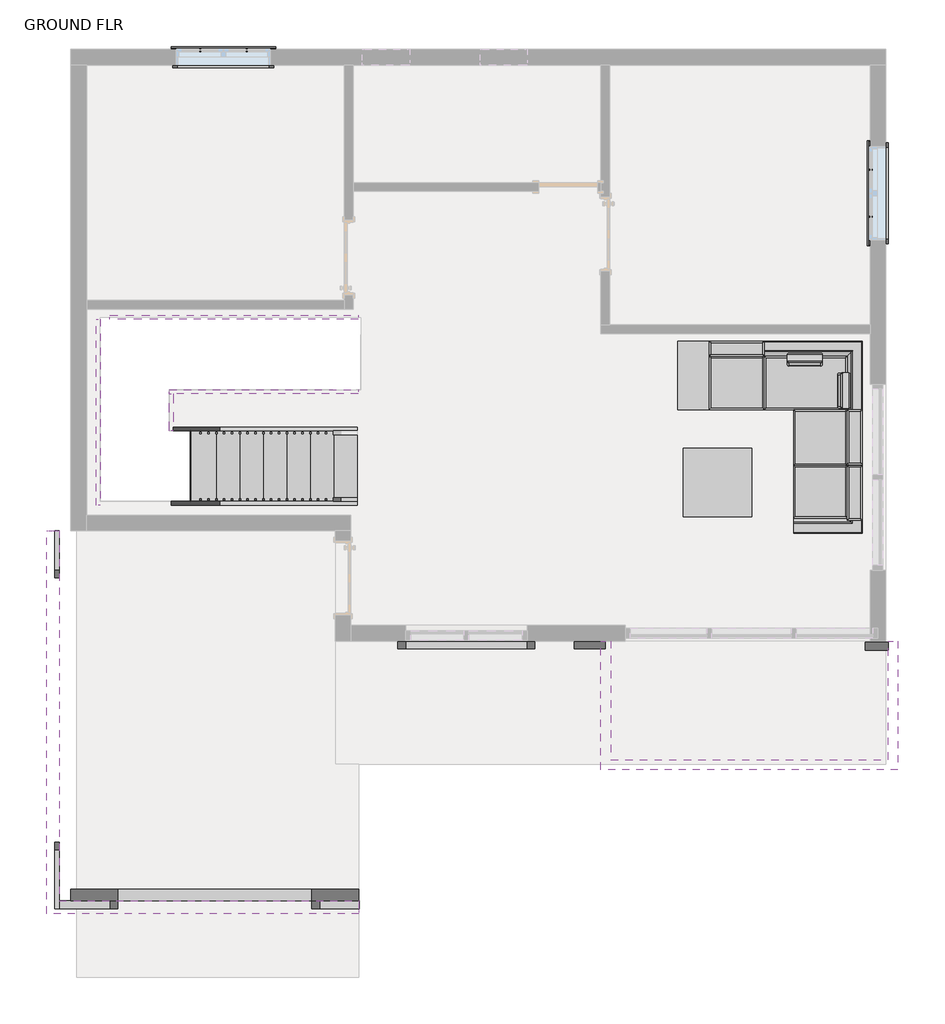
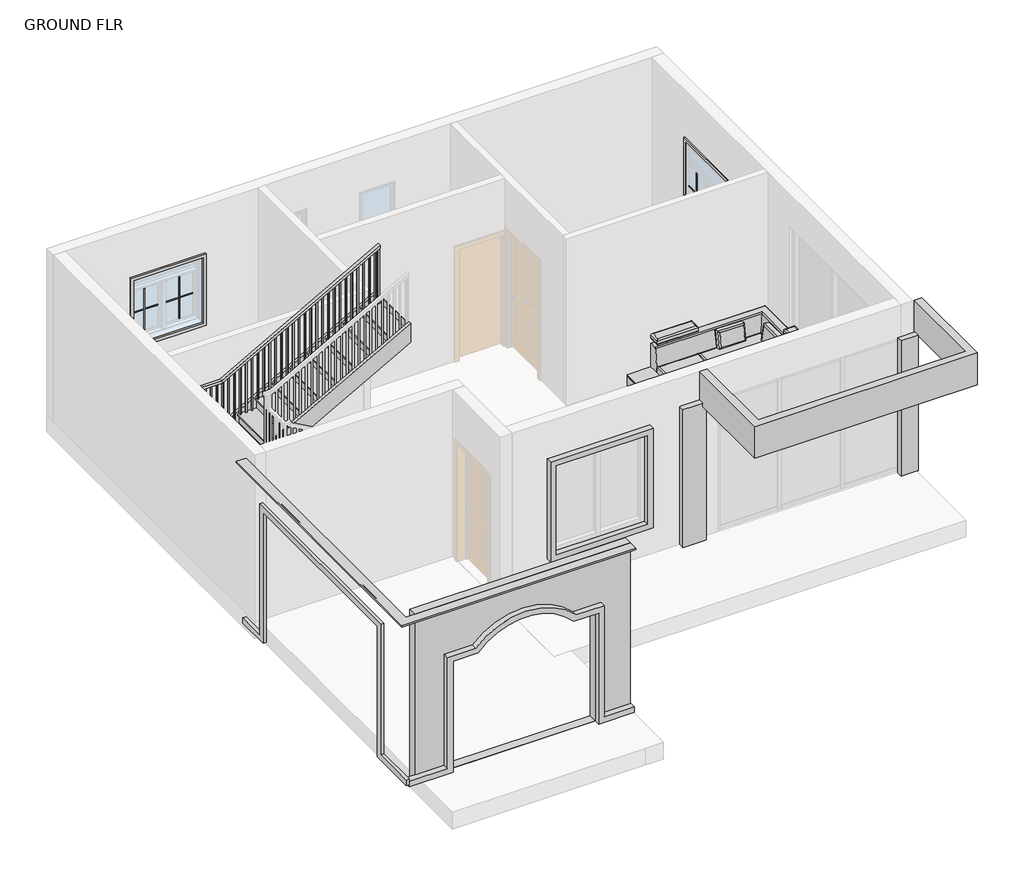
# One storey, part 3 of 3: 17 proxies, 6 members, 1 railing, 1 stair flight.
"""IFC4 building model written with IfcOpenShell, lengths in millimetres."""

from ifc_helpers import new_model, si_unit, frame, origin, place, context, project, spatial, polyline, outline, extrude, faceted_brep, transform, mapped, element, save
from components import generic_models_1_generic_models_1_99b3fc70, generic_models_10_generic_models_10_d7661e71, generic_models_11_generic_models_11_c52e9c8d, generic_models_2_generic_models_2_85994228, generic_models_3_generic_models_3_794cf474, generic_models_4_generic_models_4_3df0761b, generic_models_7_generic_models_7_ebfadceb, generic_models_9_generic_models_9_ba76ca7f, muntin_pattern_2x2_muntin_pattern_2x2_2357e71d, muntin_pattern_2x2_muntin_pattern_2x2_302d8f29, trim_window_exterior_flat_with_sill_7cfdd449, trim_window_exterior_flat_with_sill_ac84ebb5, trim_window_interior_flat_picture_frame_f1e0b15b, trim_window_interior_flat_picture_frame_caf2db4f, sectional_sofa_6482_sectional_sofa_6482_559db2f0, sectional_sofa_6482_sectional_sofa_6482_9496661e, stair_flight_1ef6648f

model = new_model("IFC4")

# Units and contexts
model_context = context("Model", 3, world=origin())
ifc_project = project(units=[si_unit("LENGTHUNIT", "METRE", prefix="MILLI")], contexts=[model_context])

# Site, building, storey
site = spatial("IfcSite", under=ifc_project)
building = spatial("IfcBuilding", under=site)
storey = spatial("IfcBuildingStorey", under=building, Name="GROUND FLR", Elevation=304.8)

# Proxies
placement = place(None, origin())
generic_models_1_generic_models_1_shape = generic_models_1_generic_models_1_99b3fc70(model_context)
element("IfcBuildingElementProxy", 1, Name="Generic Models 1 : Generic Models 1", ObjectType="Generic Models 1 : Generic Models 1", at=placement, inside=storey, context=model_context, shape_type="MappedRepresentation", body=[
    mapped(generic_models_1_generic_models_1_shape, transform((0.0, 0.0, 0.0), x_axis=(1.0, 0.0, 0.0), y_axis=(0.0, 1.0, 0.0), z_axis=(0.0, 0.0, 1.0))),
])
generic_models_10_generic_models_10_shape = generic_models_10_generic_models_10_d7661e71(model_context)
element("IfcBuildingElementProxy", 2, Name="Generic Models 10 : Generic Models 10", ObjectType="Generic Models 10 : Generic Models 10", at=placement, inside=storey, context=model_context, shape_type="MappedRepresentation", body=[
    mapped(generic_models_10_generic_models_10_shape, transform((0.0, 0.0, 0.0), x_axis=(1.0, 0.0, 0.0), y_axis=(0.0, 1.0, 0.0), z_axis=(0.0, 0.0, 1.0))),
])
generic_models_11_generic_models_11_shape = generic_models_11_generic_models_11_c52e9c8d(model_context)
element("IfcBuildingElementProxy", 3, Name="Generic Models 11 : Generic Models 11", ObjectType="Generic Models 11 : Generic Models 11", at=placement, inside=storey, context=model_context, shape_type="MappedRepresentation", body=[
    mapped(generic_models_11_generic_models_11_shape, transform((0.0, 0.0, 0.0), x_axis=(1.0, 0.0, 0.0), y_axis=(0.0, 1.0, 0.0), z_axis=(0.0, 0.0, 1.0))),
])
generic_models_2_generic_models_2_shape = generic_models_2_generic_models_2_85994228(model_context)
element("IfcBuildingElementProxy", 4, Name="Generic Models 2 : Generic Models 2", ObjectType="Generic Models 2 : Generic Models 2", at=placement, inside=storey, context=model_context, shape_type="MappedRepresentation", body=[
    mapped(generic_models_2_generic_models_2_shape, transform((0.0, 0.0, 0.0), x_axis=(1.0, 0.0, 0.0), y_axis=(0.0, 1.0, 0.0), z_axis=(0.0, 0.0, 1.0))),
])
generic_models_3_generic_models_3_shape = generic_models_3_generic_models_3_794cf474(model_context)
element("IfcBuildingElementProxy", 5, Name="Generic Models 3 : Generic Models 3", ObjectType="Generic Models 3 : Generic Models 3", at=placement, inside=storey, context=model_context, shape_type="MappedRepresentation", body=[
    mapped(generic_models_3_generic_models_3_shape, transform((0.0, 0.0, 0.0), x_axis=(1.0, 0.0, 0.0), y_axis=(0.0, 1.0, 0.0), z_axis=(0.0, 0.0, 1.0))),
])
generic_models_4_generic_models_4_shape = generic_models_4_generic_models_4_3df0761b(model_context)
element("IfcBuildingElementProxy", 6, Name="Generic Models 4 : Generic Models 4", ObjectType="Generic Models 4 : Generic Models 4", at=placement, inside=storey, context=model_context, shape_type="MappedRepresentation", body=[
    mapped(generic_models_4_generic_models_4_shape, transform((0.0, 0.0, 0.0), x_axis=(1.0, 0.0, 0.0), y_axis=(0.0, 1.0, 0.0), z_axis=(0.0, 0.0, 1.0))),
])
generic_models_7_generic_models_7_shape = generic_models_7_generic_models_7_ebfadceb(model_context)
element("IfcBuildingElementProxy", 7, Name="Generic Models 7 : Generic Models 7", ObjectType="Generic Models 7 : Generic Models 7", at=placement, inside=storey, context=model_context, shape_type="MappedRepresentation", body=[
    mapped(generic_models_7_generic_models_7_shape, transform((0.0, 0.0, 0.0), x_axis=(1.0, 0.0, 0.0), y_axis=(0.0, 1.0, 0.0), z_axis=(0.0, 0.0, 1.0))),
])
generic_models_9_generic_models_9_shape = generic_models_9_generic_models_9_ba76ca7f(model_context)
element("IfcBuildingElementProxy", 8, Name="Generic Models 9 : Generic Models 9", ObjectType="Generic Models 9 : Generic Models 9", at=placement, inside=storey, context=model_context, shape_type="MappedRepresentation", body=[
    mapped(generic_models_9_generic_models_9_shape, transform((0.0, 0.0, 0.0), x_axis=(1.0, 0.0, 0.0), y_axis=(0.0, 1.0, 0.0), z_axis=(0.0, 0.0, 1.0))),
])
muntin_pattern_2x2_muntin_pattern_2x2_shape = muntin_pattern_2x2_muntin_pattern_2x2_2357e71d(model_context)
element("IfcBuildingElementProxy", 9, Name="Muntin Pattern_2x2 : Muntin Pattern_2x2", ObjectType="Muntin Pattern_2x2 : Muntin Pattern_2x2", at=placement, inside=storey, context=model_context, shape_type="MappedRepresentation", body=[
    mapped(muntin_pattern_2x2_muntin_pattern_2x2_shape, transform((-9970.7895642, -2610.1146616, 1289.05), x_axis=(1.0, 0.0, 0.0), y_axis=(0.0, 1.0, 0.0), z_axis=(0.0, 0.0, 1.0))),
])
element("IfcBuildingElementProxy", 10, Name="Muntin Pattern_2x2 : Muntin Pattern_2x2", ObjectType="Muntin Pattern_2x2 : Muntin Pattern_2x2", at=placement, inside=storey, context=model_context, shape_type="MappedRepresentation", body=[
    mapped(muntin_pattern_2x2_muntin_pattern_2x2_shape, transform((-1272.9986584, -4768.3196866, 1289.05), x_axis=(0.0, 1.0, 0.0), y_axis=(-1.0, 0.0, 0.0), z_axis=(0.0, 0.0, 1.0))),
])
muntin_pattern_2x2_muntin_pattern_2x2_2_shape = muntin_pattern_2x2_muntin_pattern_2x2_302d8f29(model_context)
element("IfcBuildingElementProxy", 11, Name="Muntin Pattern_2x2 : Muntin Pattern_2x2", ObjectType="Muntin Pattern_2x2 : Muntin Pattern_2x2", at=placement, inside=storey, context=model_context, shape_type="MappedRepresentation", body=[
    mapped(muntin_pattern_2x2_muntin_pattern_2x2_2_shape, transform((-9364.3645642, -2610.1146616, 1289.05), x_axis=(-1.0, 0.0, 0.0), y_axis=(0.0, -1.0, 0.0), z_axis=(0.0, 0.0, 1.0))),
])
element("IfcBuildingElementProxy", 12, Name="Muntin Pattern_2x2 : Muntin Pattern_2x2", ObjectType="Muntin Pattern_2x2 : Muntin Pattern_2x2", at=placement, inside=storey, context=model_context, shape_type="MappedRepresentation", body=[
    mapped(muntin_pattern_2x2_muntin_pattern_2x2_2_shape, transform((-1272.9986584, -4161.8946866, 1289.05), x_axis=(0.0, -1.0, 0.0), y_axis=(1.0, 0.0, 0.0), z_axis=(0.0, 0.0, 1.0))),
])
trim_window_exterior_flat_with_sill_shape = trim_window_exterior_flat_with_sill_7cfdd449(model_context)
element("IfcBuildingElementProxy", 13, Name="Trim-Window-Exterior-Flat : with Sill", ObjectType="Trim-Window-Exterior-Flat : with Sill", at=placement, inside=storey, context=model_context, shape_type="MappedRepresentation", body=[
    mapped(trim_window_exterior_flat_with_sill_shape, transform((-9667.5770642, -2600.5896616, 2438.4), x_axis=(-1.0, 0.0, 0.0), y_axis=(0.0, 0.0, 1.0), z_axis=(0.0, 1.0, 0.0))),
])
trim_window_exterior_flat_with_sill_2_shape = trim_window_exterior_flat_with_sill_ac84ebb5(model_context)
element("IfcBuildingElementProxy", 14, Name="Trim-Window-Exterior-Flat : with Sill", ObjectType="Trim-Window-Exterior-Flat : with Sill", at=placement, inside=storey, context=model_context, shape_type="MappedRepresentation", body=[
    mapped(trim_window_exterior_flat_with_sill_2_shape, transform((-1282.5236584, -4465.1071866, 2438.4), x_axis=(0.0, 1.0, 0.0), y_axis=(0.0, 0.0, -1.0), z_axis=(-1.0, 0.0, 0.0))),
])
trim_window_interior_flat_picture_frame_shape = trim_window_interior_flat_picture_frame_f1e0b15b(model_context)
element("IfcBuildingElementProxy", 15, Name="Trim-Window-Interior-Flat : Picture Frame", ObjectType="Trim-Window-Interior-Flat : Picture Frame", at=placement, inside=storey, context=model_context, shape_type="MappedRepresentation", body=[
    mapped(trim_window_interior_flat_picture_frame_shape, transform((-9667.5770642, -2803.7896616, 2438.4), x_axis=(1.0, 0.0, 0.0), y_axis=(0.0, 0.0, 1.0), z_axis=(0.0, -1.0, 0.0))),
])
trim_window_interior_flat_picture_frame_2_shape = trim_window_interior_flat_picture_frame_caf2db4f(model_context)
element("IfcBuildingElementProxy", 16, Name="Trim-Window-Interior-Flat : Picture Frame", ObjectType="Trim-Window-Interior-Flat : Picture Frame", at=placement, inside=storey, context=model_context, shape_type="MappedRepresentation", body=[
    mapped(trim_window_interior_flat_picture_frame_2_shape, transform((-1079.3236584, -4465.1071866, 2438.4), x_axis=(0.0, -1.0, 0.0), y_axis=(0.0, 0.0, -1.0), z_axis=(1.0, 0.0, 0.0))),
])
sectional_sofa_6482_sectional_sofa_6482_shape = sectional_sofa_6482_sectional_sofa_6482_559db2f0(model_context)
sectional_sofa_6482_sectional_sofa_6482_2_shape = sectional_sofa_6482_sectional_sofa_6482_9496661e(model_context)
element("IfcBuildingElementProxy", 17, Name="sectional_sofa_6482 : sectional_sofa_6482", ObjectType="sectional_sofa_6482 : sectional_sofa_6482", at=placement, inside=storey, context=model_context, shape_type="MappedRepresentation", body=[
    mapped(sectional_sofa_6482_sectional_sofa_6482_shape, transform((-2654.1236584, -7674.2396616, 304.8), x_axis=(1.0, 0.0, 0.0), y_axis=(0.0, 1.0, 0.0), z_axis=(0.0, 0.0, 1.0))),
    mapped(sectional_sofa_6482_sectional_sofa_6482_2_shape, transform((-2654.1236584, -7674.2396616, 304.8), x_axis=(1.0, 0.0, 0.0), y_axis=(0.0, 1.0, 0.0), z_axis=(0.0, 0.0, 1.0))),
])

# Members
element("IfcMember", 18, ObjectType="Stringer - 2\" Width", at=placement, inside=storey, context=model_context, shape_type="SweptSolid", body=[
    extrude(outline(polyline([(304.8, -7930.9736584), (512.3983948, -7930.9736584), (1905.0, -10437.6565478), (1905.0, -11065.2781612), (304.8, -8184.9181612), (304.8, -7930.9736584)])), frame((0.0, -8512.4396616, 0.0), z_axis=(0.0, 1.0, 0.0), x_axis=(0.0, 0.0, 1.0)), (0.0, 0.0, 1.0), 50.8),
])
element("IfcMember", 19, ObjectType="Stringer - 2\" Width", at=placement, inside=storey, context=model_context, shape_type="SweptSolid", body=[
    extrude(outline(polyline([(-11264.7236584, -8512.4396616), (-11315.5236584, -8512.4396616), (-11315.5236584, -6099.4396616), (-11264.7236584, -6099.4396616), (-11264.7236584, -8512.4396616)])), frame((0.0, 0.0, 1600.2), z_axis=(0.0, 0.0, 1.0), x_axis=(1.0, 0.0, 0.0)), (0.0, 0.0, 1.0), 304.8),
])
element("IfcMember", 20, ObjectType="Stringer - 2\" Width", at=placement, inside=storey, context=model_context, shape_type="SweptSolid", body=[
    extrude(outline(polyline([(1600.2, -10517.2625614), (3042.3863873, -7921.3270642), (3391.0650614, -7921.3270642), (1600.2, -11144.8841748), (1600.2, -10517.2625614)])), frame((0.0, -6099.4396616, 0.0), z_axis=(0.0, 1.0, 0.0), x_axis=(0.0, 0.0, 1.0)), (0.0, 0.0, 1.0), 50.8),
])
element("IfcMember", 21, ObjectType="Stringer - 2\" Width", at=placement, inside=storey, context=model_context, shape_type="SweptSolid", body=[
    extrude(outline(polyline([(304.8, -7930.9736584), (512.3983948, -7930.9736584), (1838.8428392, -10318.5736584), (1490.1641651, -10318.5736584), (304.8, -8184.9181612), (304.8, -7930.9736584)])), frame((0.0, -7547.2396616, 0.0), z_axis=(0.0, 1.0, 0.0), x_axis=(0.0, 0.0, 1.0)), (0.0, 0.0, 1.0), 50.8),
])
element("IfcMember", 22, ObjectType="Stringer - 2\" Width", at=placement, inside=storey, context=model_context, shape_type="SweptSolid", body=[
    extrude(outline(polyline([(-10318.5736584, -7547.2396616), (-10369.3736584, -7547.2396616), (-10369.3736584, -7064.6396616), (-10318.5736584, -7064.6396616), (-10318.5736584, -7547.2396616)])), frame((0.0, 0.0, 1600.2), z_axis=(0.0, 0.0, 1.0), x_axis=(1.0, 0.0, 0.0)), (0.0, 0.0, 1.0), 304.8),
])
element("IfcMember", 23, ObjectType="Stringer - 2\" Width", at=placement, inside=storey, context=model_context, shape_type="SweptSolid", body=[
    extrude(outline(polyline([(2031.0391758, -10369.3736584), (1682.3605017, -10369.3736584), (3042.3863873, -7921.3270642), (3391.0650614, -7921.3270642), (2031.0391758, -10369.3736584)])), frame((0.0, -7064.6396616, 0.0), z_axis=(0.0, 1.0, 0.0), x_axis=(0.0, 0.0, 1.0)), (0.0, 0.0, 1.0), 50.8),
])

# Railing
element("IfcRailing", 24, ObjectType="Handrail - Rectangular", at=placement, inside=storey, context=model_context, shape_type="SolidModel", body=[
    faceted_brep([(-7930.9736584, -8461.6396616, 1388.5333333), (-7930.9736584, -8461.6396616, 1330.420221), (-7930.9736584, -8410.8396616, 1330.420221), (-7930.9736584, -8410.8396616, 1388.5333333), (-10369.3736584, -8461.6396616, 2743.2), (-10382.5372606, -8461.6396616, 2692.4), (-10382.5372606, -8410.8396616, 2692.4), (-10369.3736584, -8410.8396616, 2743.2), (-11264.7236584, -8461.6396616, 2743.2), (-11264.7236584, -8461.6396616, 2692.4), (-11213.9236584, -8410.8396616, 2692.4), (-11213.9236584, -8410.8396616, 2743.2), (-11264.7236584, -6099.4396616, 2743.2), (-11264.7236584, -6099.4396616, 2692.4), (-11213.9236584, -6150.2396616, 2692.4), (-11213.9236584, -6150.2396616, 2743.2), (-10664.5270642, -6099.4396616, 2743.2), (-10651.3634619, -6099.4396616, 2692.4), (-10651.3634619, -6150.2396616, 2692.4), (-10664.5270642, -6150.2396616, 2743.2), (-7921.3270642, -6099.4396616, 4267.2), (-7921.3270642, -6150.2396616, 4267.2), (-7921.3270642, -6150.2396616, 4209.0868876), (-7921.3270642, -6099.4396616, 4209.0868876)], [[[0, 1, 2, 3]], [[1, 0, 4, 5]], [[2, 1, 5, 6]], [[3, 2, 6, 7]], [[0, 3, 7, 4]], [[5, 4, 8, 9]], [[6, 5, 9, 10]], [[7, 6, 10, 11]], [[4, 7, 11, 8]], [[9, 8, 12, 13]], [[10, 9, 13, 14]], [[11, 10, 14, 15]], [[8, 11, 15, 12]], [[13, 12, 16, 17]], [[14, 13, 17, 18]], [[15, 14, 18, 19]], [[12, 15, 19, 16]], [[20, 21, 22, 23]], [[17, 16, 20, 23]], [[18, 17, 23, 22]], [[19, 18, 22, 21]], [[16, 19, 21, 20]]]),
    extrude(outline(polyline([(4166.686002, -7997.6486584), (3183.4666667, -7997.6486584), (3183.4666667, -7978.5986584), (4177.2693353, -7978.5986584), (4166.686002, -7997.6486584)])), frame((0.0, -6134.3646616, 0.0), z_axis=(0.0, 1.0, 0.0), x_axis=(0.0, 0.0, 1.0)), (0.0, 0.0, 1.0), 19.05),
    extrude(outline(polyline([(4110.2415575, -8099.2486584), (3183.4666667, -8099.2486584), (3183.4666667, -8080.1986584), (4120.8248909, -8080.1986584), (4110.2415575, -8099.2486584)])), frame((0.0, -6134.3646616, 0.0), z_axis=(0.0, 1.0, 0.0), x_axis=(0.0, 0.0, 1.0)), (0.0, 0.0, 1.0), 19.05),
    extrude(outline(polyline([(4053.7971131, -8200.8486584), (3183.4666667, -8200.8486584), (3183.4666667, -8181.7986584), (4064.3804464, -8181.7986584), (4053.7971131, -8200.8486584)])), frame((0.0, -6134.3646616, 0.0), z_axis=(0.0, 1.0, 0.0), x_axis=(0.0, 0.0, 1.0)), (0.0, 0.0, 1.0), 19.05),
    extrude(outline(polyline([(3997.3526686, -8302.4486584), (3014.1333333, -8302.4486584), (3014.1333333, -8283.3986584), (4007.936002, -8283.3986584), (3997.3526686, -8302.4486584)])), frame((0.0, -6134.3646616, 0.0), z_axis=(0.0, 1.0, 0.0), x_axis=(0.0, 0.0, 1.0)), (0.0, 0.0, 1.0), 19.05),
    extrude(outline(polyline([(3940.9082242, -8404.0486584), (3014.1333333, -8404.0486584), (3014.1333333, -8384.9986584), (3951.4915575, -8384.9986584), (3940.9082242, -8404.0486584)])), frame((0.0, -6134.3646616, 0.0), z_axis=(0.0, 1.0, 0.0), x_axis=(0.0, 0.0, 1.0)), (0.0, 0.0, 1.0), 19.05),
    extrude(outline(polyline([(3884.4637797, -8505.6486584), (3014.1333333, -8505.6486584), (3014.1333333, -8486.5986584), (3895.0471131, -8486.5986584), (3884.4637797, -8505.6486584)])), frame((0.0, -6134.3646616, 0.0), z_axis=(0.0, 1.0, 0.0), x_axis=(0.0, 0.0, 1.0)), (0.0, 0.0, 1.0), 19.05),
    extrude(outline(polyline([(3828.0193353, -8607.2486584), (2844.8, -8607.2486584), (2844.8, -8588.1986584), (3838.6026686, -8588.1986584), (3828.0193353, -8607.2486584)])), frame((0.0, -6134.3646616, 0.0), z_axis=(0.0, 1.0, 0.0), x_axis=(0.0, 0.0, 1.0)), (0.0, 0.0, 1.0), 19.05),
    extrude(outline(polyline([(3771.5748909, -8708.8486584), (2844.8, -8708.8486584), (2844.8, -8689.7986584), (3782.1582242, -8689.7986584), (3771.5748909, -8708.8486584)])), frame((0.0, -6134.3646616, 0.0), z_axis=(0.0, 1.0, 0.0), x_axis=(0.0, 0.0, 1.0)), (0.0, 0.0, 1.0), 19.05),
    extrude(outline(polyline([(3715.1304464, -8810.4486584), (2844.8, -8810.4486584), (2844.8, -8791.3986584), (3725.7137797, -8791.3986584), (3715.1304464, -8810.4486584)])), frame((0.0, -6134.3646616, 0.0), z_axis=(0.0, 1.0, 0.0), x_axis=(0.0, 0.0, 1.0)), (0.0, 0.0, 1.0), 19.05),
    extrude(outline(polyline([(3658.686002, -8912.0486584), (2675.4666667, -8912.0486584), (2675.4666667, -8892.9986584), (3669.2693353, -8892.9986584), (3658.686002, -8912.0486584)])), frame((0.0, -6134.3646616, 0.0), z_axis=(0.0, 1.0, 0.0), x_axis=(0.0, 0.0, 1.0)), (0.0, 0.0, 1.0), 19.05),
    extrude(outline(polyline([(3602.2415575, -9013.6486584), (2675.4666667, -9013.6486584), (2675.4666667, -8994.5986584), (3612.8248909, -8994.5986584), (3602.2415575, -9013.6486584)])), frame((0.0, -6134.3646616, 0.0), z_axis=(0.0, 1.0, 0.0), x_axis=(0.0, 0.0, 1.0)), (0.0, 0.0, 1.0), 19.05),
    extrude(outline(polyline([(3545.7971131, -9115.2486584), (2675.4666667, -9115.2486584), (2675.4666667, -9096.1986584), (3556.3804464, -9096.1986584), (3545.7971131, -9115.2486584)])), frame((0.0, -6134.3646616, 0.0), z_axis=(0.0, 1.0, 0.0), x_axis=(0.0, 0.0, 1.0)), (0.0, 0.0, 1.0), 19.05),
    extrude(outline(polyline([(3489.3526686, -9216.8486584), (2506.1333333, -9216.8486584), (2506.1333333, -9197.7986584), (3499.936002, -9197.7986584), (3489.3526686, -9216.8486584)])), frame((0.0, -6134.3646616, 0.0), z_axis=(0.0, 1.0, 0.0), x_axis=(0.0, 0.0, 1.0)), (0.0, 0.0, 1.0), 19.05),
    extrude(outline(polyline([(3432.9082242, -9318.4486584), (2506.1333333, -9318.4486584), (2506.1333333, -9299.3986584), (3443.4915575, -9299.3986584), (3432.9082242, -9318.4486584)])), frame((0.0, -6134.3646616, 0.0), z_axis=(0.0, 1.0, 0.0), x_axis=(0.0, 0.0, 1.0)), (0.0, 0.0, 1.0), 19.05),
    extrude(outline(polyline([(3376.4637797, -9420.0486584), (2506.1333333, -9420.0486584), (2506.1333333, -9400.9986584), (3387.0471131, -9400.9986584), (3376.4637797, -9420.0486584)])), frame((0.0, -6134.3646616, 0.0), z_axis=(0.0, 1.0, 0.0), x_axis=(0.0, 0.0, 1.0)), (0.0, 0.0, 1.0), 19.05),
    extrude(outline(polyline([(3320.0193353, -9521.6486584), (2336.8, -9521.6486584), (2336.8, -9502.5986584), (3330.6026686, -9502.5986584), (3320.0193353, -9521.6486584)])), frame((0.0, -6134.3646616, 0.0), z_axis=(0.0, 1.0, 0.0), x_axis=(0.0, 0.0, 1.0)), (0.0, 0.0, 1.0), 19.05),
    extrude(outline(polyline([(3263.5748909, -9623.2486584), (2336.8, -9623.2486584), (2336.8, -9604.1986584), (3274.1582242, -9604.1986584), (3263.5748909, -9623.2486584)])), frame((0.0, -6134.3646616, 0.0), z_axis=(0.0, 1.0, 0.0), x_axis=(0.0, 0.0, 1.0)), (0.0, 0.0, 1.0), 19.05),
    extrude(outline(polyline([(3207.1304464, -9724.8486584), (2336.8, -9724.8486584), (2336.8, -9705.7986584), (3217.7137797, -9705.7986584), (3207.1304464, -9724.8486584)])), frame((0.0, -6134.3646616, 0.0), z_axis=(0.0, 1.0, 0.0), x_axis=(0.0, 0.0, 1.0)), (0.0, 0.0, 1.0), 19.05),
    extrude(outline(polyline([(3150.686002, -9826.4486584), (2167.4666667, -9826.4486584), (2167.4666667, -9807.3986584), (3161.2693353, -9807.3986584), (3150.686002, -9826.4486584)])), frame((0.0, -6134.3646616, 0.0), z_axis=(0.0, 1.0, 0.0), x_axis=(0.0, 0.0, 1.0)), (0.0, 0.0, 1.0), 19.05),
    extrude(outline(polyline([(3094.2415575, -9928.0486584), (2167.4666667, -9928.0486584), (2167.4666667, -9908.9986584), (3104.8248909, -9908.9986584), (3094.2415575, -9928.0486584)])), frame((0.0, -6134.3646616, 0.0), z_axis=(0.0, 1.0, 0.0), x_axis=(0.0, 0.0, 1.0)), (0.0, 0.0, 1.0), 19.05),
    extrude(outline(polyline([(3037.7971131, -10029.6486584), (2167.4666667, -10029.6486584), (2167.4666667, -10010.5986584), (3048.3804464, -10010.5986584), (3037.7971131, -10029.6486584)])), frame((0.0, -6134.3646616, 0.0), z_axis=(0.0, 1.0, 0.0), x_axis=(0.0, 0.0, 1.0)), (0.0, 0.0, 1.0), 19.05),
    extrude(outline(polyline([(2981.3526686, -10131.2486584), (1998.1333333, -10131.2486584), (1998.1333333, -10112.1986584), (2991.936002, -10112.1986584), (2981.3526686, -10131.2486584)])), frame((0.0, -6134.3646616, 0.0), z_axis=(0.0, 1.0, 0.0), x_axis=(0.0, 0.0, 1.0)), (0.0, 0.0, 1.0), 19.05),
    extrude(outline(polyline([(2924.9082242, -10232.8486584), (1998.1333333, -10232.8486584), (1998.1333333, -10213.7986584), (2935.4915575, -10213.7986584), (2924.9082242, -10232.8486584)])), frame((0.0, -6134.3646616, 0.0), z_axis=(0.0, 1.0, 0.0), x_axis=(0.0, 0.0, 1.0)), (0.0, 0.0, 1.0), 19.05),
    extrude(outline(polyline([(2868.4637797, -10334.4486584), (1998.1333333, -10334.4486584), (1998.1333333, -10315.3986584), (2879.0471131, -10315.3986584), (2868.4637797, -10334.4486584)])), frame((0.0, -6134.3646616, 0.0), z_axis=(0.0, 1.0, 0.0), x_axis=(0.0, 0.0, 1.0)), (0.0, 0.0, 1.0), 19.05),
    extrude(outline(polyline([(2812.0193353, -10436.0486584), (1828.8, -10436.0486584), (1828.8, -10416.9986584), (2822.6026686, -10416.9986584), (2812.0193353, -10436.0486584)])), frame((0.0, -6134.3646616, 0.0), z_axis=(0.0, 1.0, 0.0), x_axis=(0.0, 0.0, 1.0)), (0.0, 0.0, 1.0), 19.05),
    extrude(outline(polyline([(2755.5748909, -10537.6486584), (1828.8, -10537.6486584), (1828.8, -10518.5986584), (2766.1582242, -10518.5986584), (2755.5748909, -10537.6486584)])), frame((0.0, -6134.3646616, 0.0), z_axis=(0.0, 1.0, 0.0), x_axis=(0.0, 0.0, 1.0)), (0.0, 0.0, 1.0), 19.05),
    extrude(outline(polyline([(2699.1304464, -10639.2486584), (1828.8, -10639.2486584), (1828.8, -10620.1986584), (2709.7137797, -10620.1986584), (2699.1304464, -10639.2486584)])), frame((0.0, -6134.3646616, 0.0), z_axis=(0.0, 1.0, 0.0), x_axis=(0.0, 0.0, 1.0)), (0.0, 0.0, 1.0), 19.05),
    extrude(outline(polyline([(-10740.8486584, -6115.3146616), (-10721.7986584, -6115.3146616), (-10721.7986584, -6134.3646616), (-10740.8486584, -6134.3646616), (-10740.8486584, -6115.3146616)])), frame((0.0, 0.0, 1828.8), z_axis=(0.0, 0.0, 1.0), x_axis=(1.0, 0.0, 0.0)), (0.0, 0.0, 1.0), 863.6),
    extrude(outline(polyline([(-10842.4486584, -6115.3146616), (-10823.3986584, -6115.3146616), (-10823.3986584, -6134.3646616), (-10842.4486584, -6134.3646616), (-10842.4486584, -6115.3146616)])), frame((0.0, 0.0, 1828.8), z_axis=(0.0, 0.0, 1.0), x_axis=(1.0, 0.0, 0.0)), (0.0, 0.0, 1.0), 863.6),
    extrude(outline(polyline([(-10944.0486584, -6115.3146616), (-10924.9986584, -6115.3146616), (-10924.9986584, -6134.3646616), (-10944.0486584, -6134.3646616), (-10944.0486584, -6115.3146616)])), frame((0.0, 0.0, 1828.8), z_axis=(0.0, 0.0, 1.0), x_axis=(1.0, 0.0, 0.0)), (0.0, 0.0, 1.0), 863.6),
    extrude(outline(polyline([(-11045.6486584, -6115.3146616), (-11026.5986584, -6115.3146616), (-11026.5986584, -6134.3646616), (-11045.6486584, -6134.3646616), (-11045.6486584, -6115.3146616)])), frame((0.0, 0.0, 1828.8), z_axis=(0.0, 0.0, 1.0), x_axis=(1.0, 0.0, 0.0)), (0.0, 0.0, 1.0), 863.6),
    extrude(outline(polyline([(-11147.2486584, -6115.3146616), (-11128.1986584, -6115.3146616), (-11128.1986584, -6134.3646616), (-11147.2486584, -6134.3646616), (-11147.2486584, -6115.3146616)])), frame((0.0, 0.0, 1828.8), z_axis=(0.0, 0.0, 1.0), x_axis=(1.0, 0.0, 0.0)), (0.0, 0.0, 1.0), 863.6),
    extrude(outline(polyline([(-11248.8486584, -6210.5646616), (-11248.8486584, -6191.5146616), (-11229.7986584, -6191.5146616), (-11229.7986584, -6210.5646616), (-11248.8486584, -6210.5646616)])), frame((0.0, 0.0, 1828.8), z_axis=(0.0, 0.0, 1.0), x_axis=(1.0, 0.0, 0.0)), (0.0, 0.0, 1.0), 863.6),
    extrude(outline(polyline([(-11248.8486584, -6312.1646616), (-11248.8486584, -6293.1146616), (-11229.7986584, -6293.1146616), (-11229.7986584, -6312.1646616), (-11248.8486584, -6312.1646616)])), frame((0.0, 0.0, 1828.8), z_axis=(0.0, 0.0, 1.0), x_axis=(1.0, 0.0, 0.0)), (0.0, 0.0, 1.0), 863.6),
    extrude(outline(polyline([(-11248.8486584, -6413.7646616), (-11248.8486584, -6394.7146616), (-11229.7986584, -6394.7146616), (-11229.7986584, -6413.7646616), (-11248.8486584, -6413.7646616)])), frame((0.0, 0.0, 1828.8), z_axis=(0.0, 0.0, 1.0), x_axis=(1.0, 0.0, 0.0)), (0.0, 0.0, 1.0), 863.6),
    extrude(outline(polyline([(-11248.8486584, -6515.3646616), (-11248.8486584, -6496.3146616), (-11229.7986584, -6496.3146616), (-11229.7986584, -6515.3646616), (-11248.8486584, -6515.3646616)])), frame((0.0, 0.0, 1828.8), z_axis=(0.0, 0.0, 1.0), x_axis=(1.0, 0.0, 0.0)), (0.0, 0.0, 1.0), 863.6),
    extrude(outline(polyline([(-11248.8486584, -6616.9646616), (-11248.8486584, -6597.9146616), (-11229.7986584, -6597.9146616), (-11229.7986584, -6616.9646616), (-11248.8486584, -6616.9646616)])), frame((0.0, 0.0, 1828.8), z_axis=(0.0, 0.0, 1.0), x_axis=(1.0, 0.0, 0.0)), (0.0, 0.0, 1.0), 863.6),
    extrude(outline(polyline([(-11248.8486584, -6718.5646616), (-11248.8486584, -6699.5146616), (-11229.7986584, -6699.5146616), (-11229.7986584, -6718.5646616), (-11248.8486584, -6718.5646616)])), frame((0.0, 0.0, 1828.8), z_axis=(0.0, 0.0, 1.0), x_axis=(1.0, 0.0, 0.0)), (0.0, 0.0, 1.0), 863.6),
    extrude(outline(polyline([(-11248.8486584, -6820.1646616), (-11248.8486584, -6801.1146616), (-11229.7986584, -6801.1146616), (-11229.7986584, -6820.1646616), (-11248.8486584, -6820.1646616)])), frame((0.0, 0.0, 1828.8), z_axis=(0.0, 0.0, 1.0), x_axis=(1.0, 0.0, 0.0)), (0.0, 0.0, 1.0), 863.6),
    extrude(outline(polyline([(-11248.8486584, -6921.7646616), (-11248.8486584, -6902.7146616), (-11229.7986584, -6902.7146616), (-11229.7986584, -6921.7646616), (-11248.8486584, -6921.7646616)])), frame((0.0, 0.0, 1828.8), z_axis=(0.0, 0.0, 1.0), x_axis=(1.0, 0.0, 0.0)), (0.0, 0.0, 1.0), 863.6),
    extrude(outline(polyline([(-11248.8486584, -7023.3646616), (-11248.8486584, -7004.3146616), (-11229.7986584, -7004.3146616), (-11229.7986584, -7023.3646616), (-11248.8486584, -7023.3646616)])), frame((0.0, 0.0, 1828.8), z_axis=(0.0, 0.0, 1.0), x_axis=(1.0, 0.0, 0.0)), (0.0, 0.0, 1.0), 863.6),
    extrude(outline(polyline([(-11248.8486584, -7124.9646616), (-11248.8486584, -7105.9146616), (-11229.7986584, -7105.9146616), (-11229.7986584, -7124.9646616), (-11248.8486584, -7124.9646616)])), frame((0.0, 0.0, 1828.8), z_axis=(0.0, 0.0, 1.0), x_axis=(1.0, 0.0, 0.0)), (0.0, 0.0, 1.0), 863.6),
    extrude(outline(polyline([(-11248.8486584, -7226.5646616), (-11248.8486584, -7207.5146616), (-11229.7986584, -7207.5146616), (-11229.7986584, -7226.5646616), (-11248.8486584, -7226.5646616)])), frame((0.0, 0.0, 1828.8), z_axis=(0.0, 0.0, 1.0), x_axis=(1.0, 0.0, 0.0)), (0.0, 0.0, 1.0), 863.6),
    extrude(outline(polyline([(-11248.8486584, -7328.1646616), (-11248.8486584, -7309.1146616), (-11229.7986584, -7309.1146616), (-11229.7986584, -7328.1646616), (-11248.8486584, -7328.1646616)])), frame((0.0, 0.0, 1828.8), z_axis=(0.0, 0.0, 1.0), x_axis=(1.0, 0.0, 0.0)), (0.0, 0.0, 1.0), 863.6),
    extrude(outline(polyline([(-11248.8486584, -7429.7646616), (-11248.8486584, -7410.7146616), (-11229.7986584, -7410.7146616), (-11229.7986584, -7429.7646616), (-11248.8486584, -7429.7646616)])), frame((0.0, 0.0, 1828.8), z_axis=(0.0, 0.0, 1.0), x_axis=(1.0, 0.0, 0.0)), (0.0, 0.0, 1.0), 863.6),
    extrude(outline(polyline([(-11248.8486584, -7531.3646616), (-11248.8486584, -7512.3146616), (-11229.7986584, -7512.3146616), (-11229.7986584, -7531.3646616), (-11248.8486584, -7531.3646616)])), frame((0.0, 0.0, 1828.8), z_axis=(0.0, 0.0, 1.0), x_axis=(1.0, 0.0, 0.0)), (0.0, 0.0, 1.0), 863.6),
    extrude(outline(polyline([(-11248.8486584, -7632.9646616), (-11248.8486584, -7613.9146616), (-11229.7986584, -7613.9146616), (-11229.7986584, -7632.9646616), (-11248.8486584, -7632.9646616)])), frame((0.0, 0.0, 1828.8), z_axis=(0.0, 0.0, 1.0), x_axis=(1.0, 0.0, 0.0)), (0.0, 0.0, 1.0), 863.6),
    extrude(outline(polyline([(-11248.8486584, -7734.5646616), (-11248.8486584, -7715.5146616), (-11229.7986584, -7715.5146616), (-11229.7986584, -7734.5646616), (-11248.8486584, -7734.5646616)])), frame((0.0, 0.0, 1828.8), z_axis=(0.0, 0.0, 1.0), x_axis=(1.0, 0.0, 0.0)), (0.0, 0.0, 1.0), 863.6),
    extrude(outline(polyline([(-11248.8486584, -7836.1646616), (-11248.8486584, -7817.1146616), (-11229.7986584, -7817.1146616), (-11229.7986584, -7836.1646616), (-11248.8486584, -7836.1646616)])), frame((0.0, 0.0, 1828.8), z_axis=(0.0, 0.0, 1.0), x_axis=(1.0, 0.0, 0.0)), (0.0, 0.0, 1.0), 863.6),
    extrude(outline(polyline([(-11248.8486584, -7937.7646616), (-11248.8486584, -7918.7146616), (-11229.7986584, -7918.7146616), (-11229.7986584, -7937.7646616), (-11248.8486584, -7937.7646616)])), frame((0.0, 0.0, 1828.8), z_axis=(0.0, 0.0, 1.0), x_axis=(1.0, 0.0, 0.0)), (0.0, 0.0, 1.0), 863.6),
    extrude(outline(polyline([(-11248.8486584, -8039.3646616), (-11248.8486584, -8020.3146616), (-11229.7986584, -8020.3146616), (-11229.7986584, -8039.3646616), (-11248.8486584, -8039.3646616)])), frame((0.0, 0.0, 1828.8), z_axis=(0.0, 0.0, 1.0), x_axis=(1.0, 0.0, 0.0)), (0.0, 0.0, 1.0), 863.6),
    extrude(outline(polyline([(-11248.8486584, -8140.9646616), (-11248.8486584, -8121.9146616), (-11229.7986584, -8121.9146616), (-11229.7986584, -8140.9646616), (-11248.8486584, -8140.9646616)])), frame((0.0, 0.0, 1828.8), z_axis=(0.0, 0.0, 1.0), x_axis=(1.0, 0.0, 0.0)), (0.0, 0.0, 1.0), 863.6),
    extrude(outline(polyline([(-11248.8486584, -8242.5646616), (-11248.8486584, -8223.5146616), (-11229.7986584, -8223.5146616), (-11229.7986584, -8242.5646616), (-11248.8486584, -8242.5646616)])), frame((0.0, 0.0, 1828.8), z_axis=(0.0, 0.0, 1.0), x_axis=(1.0, 0.0, 0.0)), (0.0, 0.0, 1.0), 863.6),
    extrude(outline(polyline([(-11248.8486584, -8344.1646616), (-11248.8486584, -8325.1146616), (-11229.7986584, -8325.1146616), (-11229.7986584, -8344.1646616), (-11248.8486584, -8344.1646616)])), frame((0.0, 0.0, 1828.8), z_axis=(0.0, 0.0, 1.0), x_axis=(1.0, 0.0, 0.0)), (0.0, 0.0, 1.0), 863.6),
    extrude(outline(polyline([(-11172.6486584, -8445.7646616), (-11191.6986584, -8445.7646616), (-11191.6986584, -8426.7146616), (-11172.6486584, -8426.7146616), (-11172.6486584, -8445.7646616)])), frame((0.0, 0.0, 1828.8), z_axis=(0.0, 0.0, 1.0), x_axis=(1.0, 0.0, 0.0)), (0.0, 0.0, 1.0), 863.6),
    extrude(outline(polyline([(-11071.0486584, -8445.7646616), (-11090.0986584, -8445.7646616), (-11090.0986584, -8426.7146616), (-11071.0486584, -8426.7146616), (-11071.0486584, -8445.7646616)])), frame((0.0, 0.0, 1828.8), z_axis=(0.0, 0.0, 1.0), x_axis=(1.0, 0.0, 0.0)), (0.0, 0.0, 1.0), 863.6),
    extrude(outline(polyline([(-10969.4486584, -8445.7646616), (-10988.4986584, -8445.7646616), (-10988.4986584, -8426.7146616), (-10969.4486584, -8426.7146616), (-10969.4486584, -8445.7646616)])), frame((0.0, 0.0, 1828.8), z_axis=(0.0, 0.0, 1.0), x_axis=(1.0, 0.0, 0.0)), (0.0, 0.0, 1.0), 863.6),
    extrude(outline(polyline([(-10867.8486584, -8445.7646616), (-10886.8986584, -8445.7646616), (-10886.8986584, -8426.7146616), (-10867.8486584, -8426.7146616), (-10867.8486584, -8445.7646616)])), frame((0.0, 0.0, 1828.8), z_axis=(0.0, 0.0, 1.0), x_axis=(1.0, 0.0, 0.0)), (0.0, 0.0, 1.0), 863.6),
    extrude(outline(polyline([(-10766.2486584, -8445.7646616), (-10785.2986584, -8445.7646616), (-10785.2986584, -8426.7146616), (-10766.2486584, -8426.7146616), (-10766.2486584, -8445.7646616)])), frame((0.0, 0.0, 1828.8), z_axis=(0.0, 0.0, 1.0), x_axis=(1.0, 0.0, 0.0)), (0.0, 0.0, 1.0), 863.6),
    extrude(outline(polyline([(-10664.6486584, -8445.7646616), (-10683.6986584, -8445.7646616), (-10683.6986584, -8426.7146616), (-10664.6486584, -8426.7146616), (-10664.6486584, -8445.7646616)])), frame((0.0, 0.0, 1828.8), z_axis=(0.0, 0.0, 1.0), x_axis=(1.0, 0.0, 0.0)), (0.0, 0.0, 1.0), 863.6),
    extrude(outline(polyline([(-10563.0486584, -8445.7646616), (-10582.0986584, -8445.7646616), (-10582.0986584, -8426.7146616), (-10563.0486584, -8426.7146616), (-10563.0486584, -8445.7646616)])), frame((0.0, 0.0, 1828.8), z_axis=(0.0, 0.0, 1.0), x_axis=(1.0, 0.0, 0.0)), (0.0, 0.0, 1.0), 863.6),
    extrude(outline(polyline([(-10461.4486584, -8445.7646616), (-10480.4986584, -8445.7646616), (-10480.4986584, -8426.7146616), (-10461.4486584, -8426.7146616), (-10461.4486584, -8445.7646616)])), frame((0.0, 0.0, 1828.8), z_axis=(0.0, 0.0, 1.0), x_axis=(1.0, 0.0, 0.0)), (0.0, 0.0, 1.0), 863.6),
    extrude(outline(polyline([(2690.3785543, -10378.8986584), (1828.8, -10378.8986584), (1828.8, -10359.8486584), (2679.795221, -10359.8486584), (2690.3785543, -10378.8986584)])), frame((0.0, -8445.7646616, 0.0), z_axis=(0.0, 1.0, 0.0), x_axis=(0.0, 0.0, 1.0)), (0.0, 0.0, 1.0), 19.05),
    extrude(outline(polyline([(2633.9341099, -10277.2986584), (1659.4666667, -10277.2986584), (1659.4666667, -10258.2486584), (2623.3507765, -10258.2486584), (2633.9341099, -10277.2986584)])), frame((0.0, -8445.7646616, 0.0), z_axis=(0.0, 1.0, 0.0), x_axis=(0.0, 0.0, 1.0)), (0.0, 0.0, 1.0), 19.05),
    extrude(outline(polyline([(2577.4896654, -10175.6986584), (1659.4666667, -10175.6986584), (1659.4666667, -10156.6486584), (2566.9063321, -10156.6486584), (2577.4896654, -10175.6986584)])), frame((0.0, -8445.7646616, 0.0), z_axis=(0.0, 1.0, 0.0), x_axis=(0.0, 0.0, 1.0)), (0.0, 0.0, 1.0), 19.05),
    extrude(outline(polyline([(2521.045221, -10074.0986584), (1659.4666667, -10074.0986584), (1659.4666667, -10055.0486584), (2510.4618876, -10055.0486584), (2521.045221, -10074.0986584)])), frame((0.0, -8445.7646616, 0.0), z_axis=(0.0, 1.0, 0.0), x_axis=(0.0, 0.0, 1.0)), (0.0, 0.0, 1.0), 19.05),
    extrude(outline(polyline([(2464.6007765, -9972.4986584), (1490.1333333, -9972.4986584), (1490.1333333, -9953.4486584), (2454.0174432, -9953.4486584), (2464.6007765, -9972.4986584)])), frame((0.0, -8445.7646616, 0.0), z_axis=(0.0, 1.0, 0.0), x_axis=(0.0, 0.0, 1.0)), (0.0, 0.0, 1.0), 19.05),
    extrude(outline(polyline([(2408.1563321, -9870.8986584), (1490.1333333, -9870.8986584), (1490.1333333, -9851.8486584), (2397.5729988, -9851.8486584), (2408.1563321, -9870.8986584)])), frame((0.0, -8445.7646616, 0.0), z_axis=(0.0, 1.0, 0.0), x_axis=(0.0, 0.0, 1.0)), (0.0, 0.0, 1.0), 19.05),
    extrude(outline(polyline([(2351.7118876, -9769.2986584), (1490.1333333, -9769.2986584), (1490.1333333, -9750.2486584), (2341.1285543, -9750.2486584), (2351.7118876, -9769.2986584)])), frame((0.0, -8445.7646616, 0.0), z_axis=(0.0, 1.0, 0.0), x_axis=(0.0, 0.0, 1.0)), (0.0, 0.0, 1.0), 19.05),
    extrude(outline(polyline([(2295.2674432, -9667.6986584), (1320.8, -9667.6986584), (1320.8, -9648.6486584), (2284.6841099, -9648.6486584), (2295.2674432, -9667.6986584)])), frame((0.0, -8445.7646616, 0.0), z_axis=(0.0, 1.0, 0.0), x_axis=(0.0, 0.0, 1.0)), (0.0, 0.0, 1.0), 19.05),
    extrude(outline(polyline([(2238.8229988, -9566.0986584), (1320.8, -9566.0986584), (1320.8, -9547.0486584), (2228.2396654, -9547.0486584), (2238.8229988, -9566.0986584)])), frame((0.0, -8445.7646616, 0.0), z_axis=(0.0, 1.0, 0.0), x_axis=(0.0, 0.0, 1.0)), (0.0, 0.0, 1.0), 19.05),
    extrude(outline(polyline([(2182.3785543, -9464.4986584), (1320.8, -9464.4986584), (1320.8, -9445.4486584), (2171.795221, -9445.4486584), (2182.3785543, -9464.4986584)])), frame((0.0, -8445.7646616, 0.0), z_axis=(0.0, 1.0, 0.0), x_axis=(0.0, 0.0, 1.0)), (0.0, 0.0, 1.0), 19.05),
    extrude(outline(polyline([(2125.9341099, -9362.8986584), (1151.4666667, -9362.8986584), (1151.4666667, -9343.8486584), (2115.3507765, -9343.8486584), (2125.9341099, -9362.8986584)])), frame((0.0, -8445.7646616, 0.0), z_axis=(0.0, 1.0, 0.0), x_axis=(0.0, 0.0, 1.0)), (0.0, 0.0, 1.0), 19.05),
    extrude(outline(polyline([(2069.4896654, -9261.2986584), (1151.4666667, -9261.2986584), (1151.4666667, -9242.2486584), (2058.9063321, -9242.2486584), (2069.4896654, -9261.2986584)])), frame((0.0, -8445.7646616, 0.0), z_axis=(0.0, 1.0, 0.0), x_axis=(0.0, 0.0, 1.0)), (0.0, 0.0, 1.0), 19.05),
    extrude(outline(polyline([(2013.045221, -9159.6986584), (1151.4666667, -9159.6986584), (1151.4666667, -9140.6486584), (2002.4618876, -9140.6486584), (2013.045221, -9159.6986584)])), frame((0.0, -8445.7646616, 0.0), z_axis=(0.0, 1.0, 0.0), x_axis=(0.0, 0.0, 1.0)), (0.0, 0.0, 1.0), 19.05),
    extrude(outline(polyline([(1956.6007765, -9058.0986584), (982.1333333, -9058.0986584), (982.1333333, -9039.0486584), (1946.0174432, -9039.0486584), (1956.6007765, -9058.0986584)])), frame((0.0, -8445.7646616, 0.0), z_axis=(0.0, 1.0, 0.0), x_axis=(0.0, 0.0, 1.0)), (0.0, 0.0, 1.0), 19.05),
    extrude(outline(polyline([(1900.1563321, -8956.4986584), (982.1333333, -8956.4986584), (982.1333333, -8937.4486584), (1889.5729988, -8937.4486584), (1900.1563321, -8956.4986584)])), frame((0.0, -8445.7646616, 0.0), z_axis=(0.0, 1.0, 0.0), x_axis=(0.0, 0.0, 1.0)), (0.0, 0.0, 1.0), 19.05),
    extrude(outline(polyline([(1843.7118876, -8854.8986584), (982.1333333, -8854.8986584), (982.1333333, -8835.8486584), (1833.1285543, -8835.8486584), (1843.7118876, -8854.8986584)])), frame((0.0, -8445.7646616, 0.0), z_axis=(0.0, 1.0, 0.0), x_axis=(0.0, 0.0, 1.0)), (0.0, 0.0, 1.0), 19.05),
    extrude(outline(polyline([(1787.2674432, -8753.2986584), (812.8, -8753.2986584), (812.8, -8734.2486584), (1776.6841099, -8734.2486584), (1787.2674432, -8753.2986584)])), frame((0.0, -8445.7646616, 0.0), z_axis=(0.0, 1.0, 0.0), x_axis=(0.0, 0.0, 1.0)), (0.0, 0.0, 1.0), 19.05),
    extrude(outline(polyline([(1730.8229988, -8651.6986584), (812.8, -8651.6986584), (812.8, -8632.6486584), (1720.2396654, -8632.6486584), (1730.8229988, -8651.6986584)])), frame((0.0, -8445.7646616, 0.0), z_axis=(0.0, 1.0, 0.0), x_axis=(0.0, 0.0, 1.0)), (0.0, 0.0, 1.0), 19.05),
    extrude(outline(polyline([(1674.3785543, -8550.0986584), (812.8, -8550.0986584), (812.8, -8531.0486584), (1663.795221, -8531.0486584), (1674.3785543, -8550.0986584)])), frame((0.0, -8445.7646616, 0.0), z_axis=(0.0, 1.0, 0.0), x_axis=(0.0, 0.0, 1.0)), (0.0, 0.0, 1.0), 19.05),
    extrude(outline(polyline([(1617.9341099, -8448.4986584), (643.4666667, -8448.4986584), (643.4666667, -8429.4486584), (1607.3507765, -8429.4486584), (1617.9341099, -8448.4986584)])), frame((0.0, -8445.7646616, 0.0), z_axis=(0.0, 1.0, 0.0), x_axis=(0.0, 0.0, 1.0)), (0.0, 0.0, 1.0), 19.05),
    extrude(outline(polyline([(1561.4896654, -8346.8986584), (643.4666667, -8346.8986584), (643.4666667, -8327.8486584), (1550.9063321, -8327.8486584), (1561.4896654, -8346.8986584)])), frame((0.0, -8445.7646616, 0.0), z_axis=(0.0, 1.0, 0.0), x_axis=(0.0, 0.0, 1.0)), (0.0, 0.0, 1.0), 19.05),
    extrude(outline(polyline([(1505.045221, -8245.2986584), (643.4666667, -8245.2986584), (643.4666667, -8226.2486584), (1494.4618876, -8226.2486584), (1505.045221, -8245.2986584)])), frame((0.0, -8445.7646616, 0.0), z_axis=(0.0, 1.0, 0.0), x_axis=(0.0, 0.0, 1.0)), (0.0, 0.0, 1.0), 19.05),
    extrude(outline(polyline([(1448.6007765, -8143.6986584), (474.1333333, -8143.6986584), (474.1333333, -8124.6486584), (1438.0174432, -8124.6486584), (1448.6007765, -8143.6986584)])), frame((0.0, -8445.7646616, 0.0), z_axis=(0.0, 1.0, 0.0), x_axis=(0.0, 0.0, 1.0)), (0.0, 0.0, 1.0), 19.05),
    extrude(outline(polyline([(1392.1563321, -8042.0986584), (474.1333333, -8042.0986584), (474.1333333, -8023.0486584), (1381.5729988, -8023.0486584), (1392.1563321, -8042.0986584)])), frame((0.0, -8445.7646616, 0.0), z_axis=(0.0, 1.0, 0.0), x_axis=(0.0, 0.0, 1.0)), (0.0, 0.0, 1.0), 19.05),
    extrude(outline(polyline([(-11248.8486584, -6134.3646616), (-11248.8486584, -6115.3146616), (-11229.7986584, -6115.3146616), (-11229.7986584, -6134.3646616), (-11248.8486584, -6134.3646616)])), frame((0.0, 0.0, 1828.8), z_axis=(0.0, 0.0, 1.0), x_axis=(1.0, 0.0, 0.0)), (0.0, 0.0, 1.0), 863.6),
    extrude(outline(polyline([(-11229.7986584, -8445.7646616), (-11248.8486584, -8445.7646616), (-11248.8486584, -8426.7146616), (-11229.7986584, -8426.7146616), (-11229.7986584, -8445.7646616)])), frame((0.0, 0.0, 1828.8), z_axis=(0.0, 0.0, 1.0), x_axis=(1.0, 0.0, 0.0)), (0.0, 0.0, 1.0), 863.6),
    extrude(outline(polyline([(4198.5035543, -7940.3770642), (3183.4666667, -7940.3770642), (3183.4666667, -7921.3270642), (4209.0868876, -7921.3270642), (4198.5035543, -7940.3770642)])), frame((0.0, -6134.3646616, 0.0), z_axis=(0.0, 1.0, 0.0), x_axis=(0.0, 0.0, 1.0)), (0.0, 0.0, 1.0), 19.05),
    extrude(outline(polyline([(1341.0035543, -7950.0236584), (474.1333333, -7950.0236584), (474.1333333, -7930.9736584), (1330.420221, -7930.9736584), (1341.0035543, -7950.0236584)])), frame((0.0, -8445.7646616, 0.0), z_axis=(0.0, 1.0, 0.0), x_axis=(0.0, 0.0, 1.0)), (0.0, 0.0, 1.0), 19.05),
])

# Stair flight
stair_flight_shape = stair_flight_1ef6648f(model_context)
element("IfcStairFlight", 25, ObjectType="2\" Tread 1\" Nosing 1/4\" Riser", at=placement, inside=storey, context=model_context, shape_type="MappedRepresentation", body=[
    mapped(stair_flight_shape, transform((0.0, 0.0, 0.0), x_axis=(1.0, 0.0, 0.0), y_axis=(0.0, 1.0, 0.0), z_axis=(0.0, 0.0, 1.0))),
])

save(model, "model.ifc")

# Revit data of these elements
# Type "Muntin Pattern_2x2 : Muntin Pattern_2x2"
#   Width [instance default] = 4' - 0"
#   Thickness = 0' - 0 1/2"
#   Height [instance default] = 4' - 0"
#   Distance = 0' - 0 3/4"
#   Interior Material [instance default] = none
#   Exterior Material [instance default] = none
#   Default Elevation = 0
# Type "Trim-Window-Exterior-Flat : with Sill"
#   Trim Width = 0' - 2 1/4"
#   Trim Thickness_Picture Frame = 0' - 1 1/4"
#   Trim Thickness_with Sill = 0' - 0 3/4"
#   Sill Thickness = 0' - 1 1/4"
#   Opening Width [instance default] = 2' - 0"
#   Opening Height [instance default] = 3' - 0"
#   Default Elevation = 4' - 0"
#   Sill = yes
#   Picture Frame = no
#   Trim Material [instance default] = none
# Type "Trim-Window-Interior-Flat : Picture Frame"
#   Trim Thickness_Picture Frame = 0' - 1 1/4"
#   Trim Width = 0' - 2 1/4"
#   Trim Thickness_with Sill = 0' - 0 3/4"
#   Sill Thickness = 0' - 1 1/4"
#   Opening Width [instance default] = 2' - 0"
#   Opening Height [instance default] = 3' - 0"
#   Default Elevation = 4' - 0"
#   Sill = no
#   Picture Frame = yes
#   Trim Material [instance default] = none
# Type "sectional_sofa_6482 : sectional_sofa_6482"
#   frame trim = frame trim
#   fabric = fabric
#   Frame = frame
#   FABRIC 2 = fabric 2
#   Default Elevation = 0
# Type "Handrail - Rectangular"
#   Assembly Code = "C2010400"
#   built-in parameter 1008612 = 0.0416667 (stored number, unit not read)
#   built-in parameter 1008611 = 0.0416667 (stored number, unit not read)
#   built-in parameter 1008609 = 0.333333 (stored number, unit not read)
#   built-in parameter 1008604 = 0.166667 (stored number, unit not read)
#   built-in parameter 1008603 = 0.166667 (stored number, unit not read)
#   Railing Height = 3' - 0"
#   built-in parameter 1008630 = 2
#   built-in parameter 1008610 = 2
#   built-in parameter 1008618 = Baluster - Square : 3/4"
# Element 1 (IfcBuildingElementProxy, "Generic Models 1 : Generic Models 1")
#   Phase Created = New Construction
#   Materials on its faces: "ACCENT BEIGE COLOUR"
# Element 2 (IfcBuildingElementProxy, "Generic Models 10 : Generic Models 10")
#   Phase Created = New Construction
#   Materials on its faces: "ACCENT BEIGE COLOUR"
# Element 3 (IfcBuildingElementProxy, "Generic Models 11 : Generic Models 11")
#   Phase Created = New Construction
#   Materials on its faces: "ACCENT BEIGE COLOUR"
# Element 4 (IfcBuildingElementProxy, "Generic Models 2 : Generic Models 2")
#   Phase Created = New Construction
#   Materials on its faces: "white colour"
# Element 5 (IfcBuildingElementProxy, "Generic Models 3 : Generic Models 3")
#   Phase Created = New Construction
#   Materials on its faces: "white colour"
# Element 6 (IfcBuildingElementProxy, "Generic Models 4 : Generic Models 4")
#   Phase Created = New Construction
#   Materials on its faces: "white colour"
# Element 7 (IfcBuildingElementProxy, "Generic Models 7 : Generic Models 7")
#   Phase Created = New Construction
#   Materials on its faces: "white colour"
# Element 8 (IfcBuildingElementProxy, "Generic Models 9 : Generic Models 9")
#   Phase Created = New Construction
#   Materials on its faces: "ACCENT BEIGE COLOUR"
# Elements 9, 10, 11, 12 (IfcBuildingElementProxy, "Muntin Pattern_2x2 : Muntin Pattern_2x2")
#   Width = 1' - 6 5/8"
#   Height = 2' - 6 1/2"
#   Interior Material = Wood - Stained
#   Exterior Material = Clad - White
#   Phase Created = New Construction
#   Materials on its faces: "Clad - White", "Wood - Stained"
# Elements 13, 14 (IfcBuildingElementProxy, "Trim-Window-Exterior-Flat : with Sill")
#   Opening Width = 4' - 0"
#   Opening Height = 4' - 0"
#   Trim Material = Clad - White
#   Phase Created = New Construction
#   Materials on its faces: "Clad - White"
# Elements 15, 16 (IfcBuildingElementProxy, "Trim-Window-Interior-Flat : Picture Frame")
#   Opening Width = 4' - 0"
#   Opening Height = 4' - 0"
#   Trim Material = Wood - Stained
#   Phase Created = New Construction
#   Materials on its faces: "Wood - Stained"
# Element 17 (IfcBuildingElementProxy, "sectional_sofa_6482 : sectional_sofa_6482")
#   Phase Created = New Construction
#   Materials on its faces: "frame trim", "fabric", "fabric 2", "frame"
# Elements 18, 19, 20, 21, 22, 23 (IfcMember, "Stringer - 2\" Width")
#   Phase Created = New Construction
# Element 24 (IfcRailing, "Handrail - Rectangular")
#   Phase Created = New Construction
# Element 25 (IfcStairFlight, "2\" Tread 1\" Nosing 1/4\" Riser")
#   Phase Created = New Construction
#   Materials on its faces: "MARBLE FLOORING 6\""
# Materials
#   "frame trim": class "Metal", colour RGB 182 182 182, transparency 0
#   "fabric": class "Leather", colour RGB 255 245 240, transparency 0
#   "frame": class "Wood", colour RGB 71 38 7, transparency 0
#   "fabric 2": class "Fabric", colour RGB 128 0 0, transparency 0
#   "ACCENT BEIGE COLOUR": class "Generic", colour RGB 120 120 120, transparency 0, Cost = 0
#   "white colour": class "Generic", colour RGB 120 120 120, transparency 0, Cost = 0
#   "Clad - White": class "Wood", colour RGB 242 242 238, transparency 0, Cost = 0
#   "Wood - Stained": class "Wood", colour RGB 224 178 126, transparency 0, Cost = 0
#   "MARBLE FLOORING 6\"": class "Generic", colour RGB 120 120 120, transparency 0, Cost = 0
